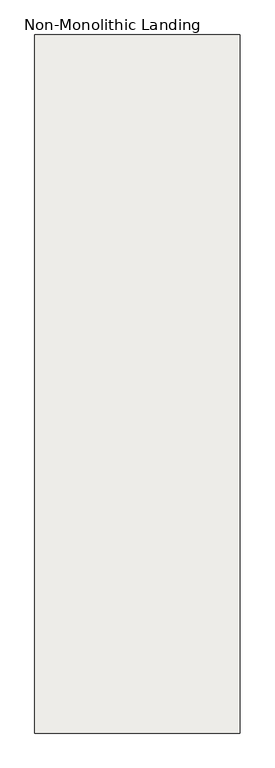
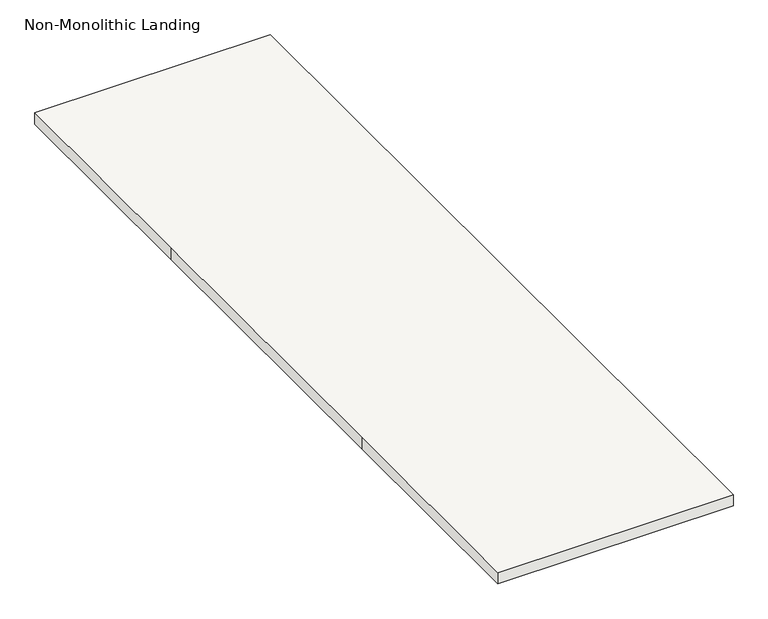
"""IFC4 building model written with IfcOpenShell, lengths in millimetres: slab geometry, Non-Monolithic Landing."""

from ifc_helpers import new_model, si_unit, frame, origin, place, context, project, spatial, polyline, outline, extrude, source, transform, mapped, element, save


def non_monolithic_landing_146c630b(model_context):
    return source(origin(), model_context, "Body", "SweptSolid", [
        extrude(outline(polyline([(4688.8435815, -2974.091395), (5688.8435815, -2974.091395), (5688.8435815, -6376.491395), (4688.8435815, -6376.491395), (4688.8435815, -5376.491395), (4688.8435815, -3974.091395), (4688.8435815, -2974.091395)])), frame((0.0, 0.0, 1600.0), z_axis=(0.0, 0.0, 1.0), x_axis=(1.0, 0.0, 0.0)), (0.0, 0.0, 1.0), 50.0),
    ])


if __name__ == "__main__":
    model = new_model("IFC4")
    model_context = context("Model", 3, world=origin())
    ifc_project = project(units=[si_unit("LENGTHUNIT", "METRE", prefix="MILLI")], contexts=[model_context])
    site = spatial("IfcSite", under=ifc_project)
    building = spatial("IfcBuilding", under=site)
    placement = place(None, origin())
    non_monolithic_landing_shape = non_monolithic_landing_146c630b(model_context)
    element("IfcSlab", 1, ObjectType="Non-Monolithic Landing", at=placement, inside=building, context=model_context, shape_type="MappedRepresentation", body=[
        mapped(non_monolithic_landing_shape, transform((0.0, 0.0, 0.0), x_axis=(1.0, 0.0, 0.0), y_axis=(0.0, 1.0, 0.0), z_axis=(0.0, 0.0, 1.0))),
    ])
    save(model, "model.ifc")
